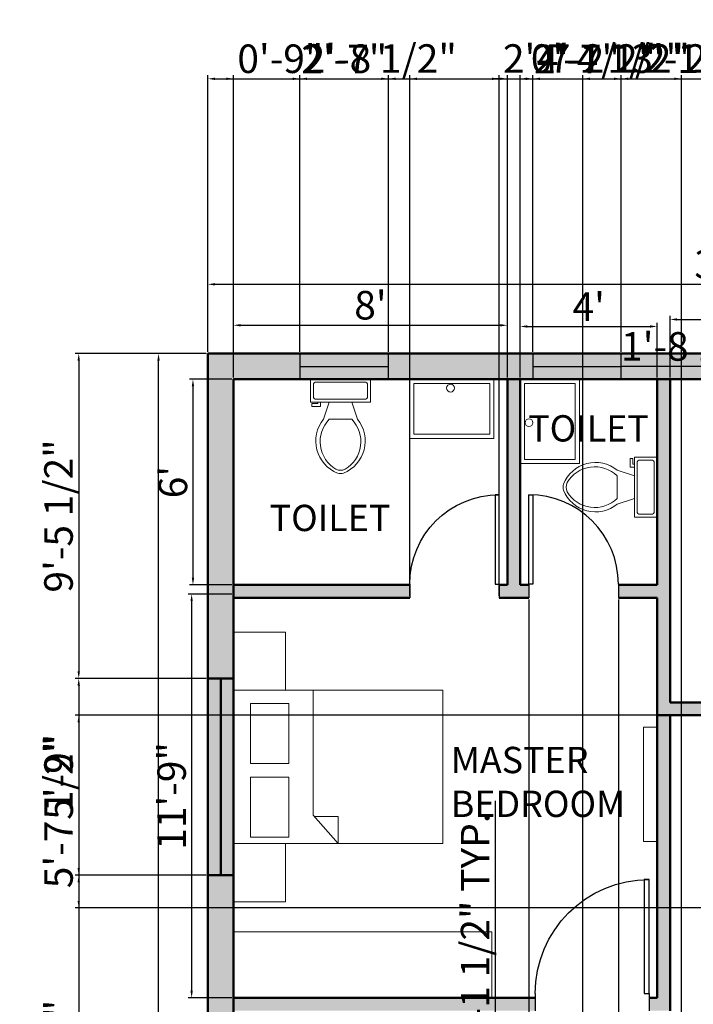
# Model space of a CAD drawing. Units: inches. Extents: x 1344 to 2521, y 3236 to 4924.
# Tile 11 of 14: x 1348 to 1584, y 4525 to 4870. Entities that reach past the tile are written whole.
import ezdxf

# ---------------------------------------------------------------- set-up
doc = ezdxf.new("R2010")
doc.units = ezdxf.units.IN
for name, color, linetype, lineweight in [('A-ANNO-DIMS', 2, 'Continuous', 18), ('A-AREA-IDEN', 3, 'Continuous', 18), ('A-DOOR', 50, 'Continuous', 25), ('A-FLOR-FIXT', 8, 'Continuous', 18), ('A-FURN', 130, 'Continuous', 18), ('A-GLAZ', 150, 'Continuous', 25), ('A-WALL', 31, 'Continuous', 50), ('A-WALL-PATT', 8, 'Continuous', 13)]:
    doc.layers.add(name, color=color, linetype=linetype, lineweight=lineweight)
doc.styles.get("Standard").update_dxf_attribs({"font": 'arial.ttf'})
doc.dimstyles.new('ISO-25', dxfattribs={"dimtxt": 10, "dimasz": 2.5, "dimexe": 1.25, "dimexo": 0.625, "dimtad": 1, "dimdec": 0, "dimlunit": 4, "dimtxsty": 'Standard', "dimcen": 2.5, "dimadec": 0, "dimazin": 0, "dimtfac": 1, "dimtdec": 0, "dimtmove": 0, "dimatfit": 3, "dimfxl": 1, "dimarcsym": 0})

# ---------------------------------------------------------------- blocks, each defined once
blk = doc.blocks.new('*U6')
for p, q in [((9.5, -6), (9.5, -2)), ((-10, -8.5), (-8, -8.5)), ((-10, -9.5), (-10, -8.5)), ((-7, -9.5), (-10, -9.5)), ((-8, -8.5), (-8, -8)), ((-7, -8), (-7, -9.5)), ((-4, -8), (-6, -14)), ((4, -8), (6, -14)), ((4, -14), (-4, -14))]:
    blk.add_line(p, q)
blk.add_lwpolyline([(10.5, -8), (10.5, 0), (-10.5, 0), (-10.5, -8)], close=True)
for points in [[(-9.5, -2), (-9.5, -6)], [(8.5, -1), (-8.5, -1)], [(-8.5, -7), (8.5, -7)]]:
    blk.add_lwpolyline(points)
for centre, radius, start, end in [((-8.62, -1.88), 0.884, 81.8699, 188.1301), ((8.62, -1.88), 0.884, 351.8699, 98.1301), ((-8.62, -6.12), 0.884, 171.8699, 278.1301), ((8.62, -6.12), 0.884, 261.8699, 8.1301), ((3.52, -21.58), 12.17, 141.4691, 247.9714), ((4.2, -21.82), 11.33, 136.3677, 238.9468), ((-3.52, -21.58), 12.17, 292.0284, 38.5307), ((-4.2, -21.82), 11.33, 301.053, 43.6321), ((0, -27.88), 4, 245.7318, 294.2682), ((0, -29), 4, 254.8605, 285.1395)]:
    blk.add_arc(centre, radius, start, end)
blk = doc.blocks.new('*U2')
for p, q in [((0, 0), (0, -6)), ((40, 0), (40, -6))]:
    blk.add_line(p, q)
blk.add_lwpolyline([(0, 0), (0, 40), (1.75, 40), (1.75, 0)], close=True)
blk.add_arc((0, 0), 40, 0, 90)
blk = doc.blocks.new('*D15')
at = {"layer": 'A-ANNO-DIMS', "color": 0, "lineweight": -2, "transparency": 16777216}
for p, q in [((1413.52, 4753.84), (1413.52, 4778.73)), ((1416.02, 4777.48), (1771.02, 4777.48)), ((1773.52, 4753.84), (1773.52, 4778.73))]:
    blk.add_line(p, q, dxfattribs=at)
at = {"layer": 'A-ANNO-DIMS', "color": 0, "lineweight": 100, "transparency": 16777216}
for points in [[(1416.02, 4777.9), (1416.02, 4777.06), (1413.52, 4777.48)], [(1771.02, 4777.9), (1771.02, 4777.06), (1773.52, 4777.48)]]:
    blk.add_solid(points, dxfattribs=at)
at = {"layer": 'Defpoints', "color": 0, "lineweight": 100, "transparency": 16777216}
for p in [(1773.52, 4777.48), (1413.52, 4753.21), (1773.52, 4753.21)]:
    blk.add_point(p, dxfattribs=at)
at = {"layer": 'A-ANNO-DIMS', "color": 0, "transparency": 16777216, "insert": (1593.52, 4783.21), "char_height": 10, "attachment_point": 5}
blk.add_mtext("30'", dxfattribs=at)
blk = doc.blocks.new('*D16')
at = {"layer": 'A-ANNO-DIMS', "color": 0, "lineweight": -2, "transparency": 16777216}
for p, q in [((1412.89, 4753.21), (1394.98, 4753.21)), ((1396.23, 4155.71), (1396.23, 4750.71)), ((1412.89, 4153.21), (1394.98, 4153.21))]:
    blk.add_line(p, q, dxfattribs=at)
at = {"layer": 'A-ANNO-DIMS', "color": 0, "lineweight": 100, "transparency": 16777216}
for points in [[(1395.81, 4750.71), (1396.65, 4750.71), (1396.23, 4753.21)], [(1395.81, 4155.71), (1396.65, 4155.71), (1396.23, 4153.21)]]:
    blk.add_solid(points, dxfattribs=at)
at = {"layer": 'Defpoints', "color": 0, "lineweight": 100, "transparency": 16777216}
for p in [(1396.23, 4753.21), (1413.52, 4753.21), (1413.52, 4153.21)]:
    blk.add_point(p, dxfattribs=at)
at = {"layer": 'A-ANNO-DIMS', "color": 0, "transparency": 16777216, "insert": (1390.5, 4453.21), "char_height": 10, "attachment_point": 5, "rotation": 90}
blk.add_mtext("50'", dxfattribs=at)
blk = doc.blocks.new('*D17')
at = {"layer": 'A-ANNO-DIMS', "color": 0, "lineweight": -2, "transparency": 16777216}
for p, q in [((1422.52, 4744.84), (1422.52, 4764.39)), ((1425.02, 4763.14), (1516.02, 4763.14)), ((1518.52, 4744.84), (1518.52, 4764.39))]:
    blk.add_line(p, q, dxfattribs=at)
at = {"layer": 'A-ANNO-DIMS', "color": 0, "lineweight": 100, "transparency": 16777216}
for points in [[(1425.02, 4763.55), (1425.02, 4762.72), (1422.52, 4763.14)], [(1516.02, 4763.55), (1516.02, 4762.72), (1518.52, 4763.14)]]:
    blk.add_solid(points, dxfattribs=at)
at = {"layer": 'Defpoints', "color": 0, "lineweight": 100, "transparency": 16777216}
for p in [(1518.52, 4763.14), (1422.52, 4744.21), (1518.52, 4744.21)]:
    blk.add_point(p, dxfattribs=at)
at = {"layer": 'A-ANNO-DIMS', "color": 0, "transparency": 16777216, "insert": (1470.52, 4768.87), "char_height": 10, "attachment_point": 5}
blk.add_mtext("8'", dxfattribs=at)
blk = doc.blocks.new('*D18')
at = {"layer": 'A-ANNO-DIMS', "color": 0, "lineweight": -2, "transparency": 16777216}
for p, q in [((1523.02, 4744.84), (1523.02, 4763.97)), ((1525.52, 4762.72), (1568.52, 4762.72)), ((1571.02, 4744.84), (1571.02, 4763.97))]:
    blk.add_line(p, q, dxfattribs=at)
at = {"layer": 'A-ANNO-DIMS', "color": 0, "lineweight": 100, "transparency": 16777216}
for points in [[(1525.52, 4763.14), (1525.52, 4762.3), (1523.02, 4762.72)], [(1568.52, 4763.14), (1568.52, 4762.3), (1571.02, 4762.72)]]:
    blk.add_solid(points, dxfattribs=at)
at = {"layer": 'Defpoints', "color": 0, "lineweight": 100, "transparency": 16777216}
for p in [(1571.02, 4762.72), (1523.02, 4744.21), (1571.02, 4744.21)]:
    blk.add_point(p, dxfattribs=at)
at = {"layer": 'A-ANNO-DIMS', "color": 0, "transparency": 16777216, "insert": (1547.02, 4768.34), "char_height": 10, "attachment_point": 5}
blk.add_mtext("4'", dxfattribs=at)
blk = doc.blocks.new('*D19')
at = {"layer": 'A-ANNO-DIMS', "color": 0, "lineweight": -2, "transparency": 16777216}
for p, q in [((1575.52, 4744.84), (1575.52, 4766.43)), ((1640.94, 4744.84), (1640.94, 4766.43)), ((1578.02, 4765.18), (1638.44, 4765.18))]:
    blk.add_line(p, q, dxfattribs=at)
at = {"layer": 'A-ANNO-DIMS', "color": 0, "lineweight": 100, "transparency": 16777216}
for points in [[(1578.02, 4765.59), (1578.02, 4764.76), (1575.52, 4765.18)], [(1638.44, 4765.59), (1638.44, 4764.76), (1640.94, 4765.18)]]:
    blk.add_solid(points, dxfattribs=at)
at = {"layer": 'Defpoints', "color": 0, "lineweight": 100, "transparency": 16777216}
for p in [(1640.94, 4765.18), (1575.52, 4744.21), (1640.94, 4744.21)]:
    blk.add_point(p, dxfattribs=at)
at = {"layer": 'A-ANNO-DIMS', "color": 0, "transparency": 16777216, "insert": (1608.23, 4770.89), "char_height": 10, "attachment_point": 5}
blk.add_mtext('5\'-5"', dxfattribs=at)
blk = doc.blocks.new('*D21')
at = {"layer": 'A-ANNO-DIMS', "color": 0, "lineweight": -2, "transparency": 16777216}
for p, q in [((1421.89, 4744.21), (1407.05, 4744.21)), ((1408.3, 4741.71), (1408.3, 4674.71)), ((1421.89, 4672.21), (1407.05, 4672.21))]:
    blk.add_line(p, q, dxfattribs=at)
at = {"layer": 'A-ANNO-DIMS', "color": 0, "lineweight": 100, "transparency": 16777216}
for points in [[(1407.89, 4741.71), (1408.72, 4741.71), (1408.3, 4744.21)], [(1407.89, 4674.71), (1408.72, 4674.71), (1408.3, 4672.21)]]:
    blk.add_solid(points, dxfattribs=at)
at = {"layer": 'Defpoints', "color": 0, "lineweight": 100, "transparency": 16777216}
for p in [(1422.52, 4744.21), (1408.3, 4672.21), (1422.52, 4672.21)]:
    blk.add_point(p, dxfattribs=at)
at = {"layer": 'A-ANNO-DIMS', "color": 0, "transparency": 16777216, "insert": (1402.57, 4708.21), "char_height": 10, "attachment_point": 5, "rotation": 90}
blk.add_mtext("6'", dxfattribs=at)
blk = doc.blocks.new('*D22')
at = {"layer": 'A-ANNO-DIMS', "color": 0, "lineweight": -2, "transparency": 16777216}
for p, q in [((1421.89, 4669), (1406.59, 4669)), ((1407.84, 4666.5), (1407.84, 4530.04)), ((1421.89, 4527.54), (1406.59, 4527.54))]:
    blk.add_line(p, q, dxfattribs=at)
at = {"layer": 'A-ANNO-DIMS', "color": 0, "lineweight": 100, "transparency": 16777216}
for points in [[(1407.42, 4666.5), (1408.25, 4666.5), (1407.84, 4669)], [(1407.42, 4530.04), (1408.25, 4530.04), (1407.84, 4527.54)]]:
    blk.add_solid(points, dxfattribs=at)
at = {"layer": 'Defpoints', "color": 0, "lineweight": 100, "transparency": 16777216}
for p in [(1422.52, 4669), (1407.84, 4527.54), (1422.52, 4527.54)]:
    blk.add_point(p, dxfattribs=at)
at = {"layer": 'A-ANNO-DIMS', "color": 0, "transparency": 16777216, "insert": (1402.11, 4598.27), "char_height": 10, "attachment_point": 5, "rotation": 90}
blk.add_mtext('11\'-9"', dxfattribs=at)
blk = doc.blocks.new('BED-DOUBLE')
for p, q in [((27.95, 53.78), (27.95, 9.98)), ((27.95, 9.98), (36.68, 0)), ((36.68, 9.56), (28.32, 9.56)), ((36.68, 0), (36.68, 9.56))]:
    blk.add_line(p, q)
for points in [[(0, 0), (73.35, 0), (73.35, 53.78), (0, 53.78)], [(5.91, 28.08), (19.39, 28.08), (19.39, 49.13), (5.91, 49.13)], [(5.91, 2.27), (19.39, 2.27), (19.39, 23.31), (5.91, 23.31)]]:
    blk.add_lwpolyline(points, close=True)
blk = doc.blocks.new('WASH-BASIN')
for points in [[(29.51, 20.73), (0, 20.73), (0, 0), (29.51, 0)], [(28.05, 19.27), (1.46, 19.27), (1.46, 1.46), (28.05, 1.46)]]:
    blk.add_lwpolyline(points, close=True)
blk.add_circle((14.31, 17.66), 1.38)
blk = doc.blocks.new('*D63')
at = {"layer": 'A-ANNO-DIMS', "color": 0, "lineweight": -2, "transparency": 16777216}
for p, q in [((1514.3, 4415.14), (1514.3, 4596.59)), ((1503.92, 4415.14), (1515.55, 4415.14)), ((1514.3, 4344.29), (1514.3, 4412.64)), ((1503.92, 4341.79), (1515.55, 4341.79))]:
    blk.add_line(p, q, dxfattribs=at)
at = {"layer": 'A-ANNO-DIMS', "color": 0, "lineweight": 100, "transparency": 16777216}
for points in [[(1513.88, 4412.64), (1514.72, 4412.64), (1514.3, 4415.14)], [(1513.88, 4344.29), (1514.72, 4344.29), (1514.3, 4341.79)]]:
    blk.add_solid(points, dxfattribs=at)
at = {"layer": 'Defpoints', "color": 0, "lineweight": 100, "transparency": 16777216}
for p in [(1503.3, 4415.14), (1514.3, 4415.14), (1503.3, 4341.79)]:
    blk.add_point(p, dxfattribs=at)
at = {"layer": 'A-ANNO-DIMS', "color": 0, "transparency": 16777216, "insert": (1508.5, 4507.12), "char_height": 10, "attachment_point": 5, "rotation": 90}
blk.add_mtext('DOUBLE BED 6\'-1 1/2" TYP.', dxfattribs=at)
blk = doc.blocks.new('*D66')
at = {"layer": 'A-ANNO-DIMS', "color": 0, "lineweight": -2, "transparency": 16777216}
for p, q in [((1645.44, 4744.84), (1645.44, 4749.89)), ((1666.17, 4744.84), (1666.17, 4749.89)), ((1645.44, 4748.64), (1558.38, 4748.64)), ((1663.67, 4748.64), (1647.94, 4748.64))]:
    blk.add_line(p, q, dxfattribs=at)
at = {"layer": 'A-ANNO-DIMS', "color": 0, "lineweight": 100, "transparency": 16777216}
for points in [[(1647.94, 4749.05), (1647.94, 4748.22), (1645.44, 4748.64)], [(1663.67, 4749.05), (1663.67, 4748.22), (1666.17, 4748.64)]]:
    blk.add_solid(points, dxfattribs=at)
at = {"layer": 'Defpoints', "color": 0, "lineweight": 100, "transparency": 16777216}
for p in [(1645.44, 4748.64), (1645.44, 4744.21), (1666.17, 4744.21)]:
    blk.add_point(p, dxfattribs=at)
at = {"layer": 'A-ANNO-DIMS', "color": 0, "transparency": 16777216, "insert": (1600.66, 4754.43), "char_height": 10, "attachment_point": 5}
blk.add_mtext('1\'-8 1/2" TYP.', dxfattribs=at)
blk = doc.blocks.new('*D69')
at = {"layer": 'A-ANNO-DIMS', "color": 0, "lineweight": -2, "transparency": 16777216}
for p, q in [((1413.52, 4753.84), (1413.52, 4850.71)), ((1416.02, 4849.46), (1420.02, 4849.46)), ((1422.52, 4744.84), (1422.52, 4850.71)), ((1422.52, 4849.46), (1452.85, 4849.46))]:
    blk.add_line(p, q, dxfattribs=at)
at = {"layer": 'A-ANNO-DIMS', "color": 0, "lineweight": 100, "transparency": 16777216}
for points in [[(1416.02, 4849.88), (1416.02, 4849.04), (1413.52, 4849.46)], [(1420.02, 4849.88), (1420.02, 4849.04), (1422.52, 4849.46)]]:
    blk.add_solid(points, dxfattribs=at)
at = {"layer": 'Defpoints', "color": 0, "lineweight": 100, "transparency": 16777216}
for p in [(1422.52, 4849.46), (1413.52, 4753.21), (1422.52, 4744.21)]:
    blk.add_point(p, dxfattribs=at)
at = {"layer": 'A-ANNO-DIMS', "color": 0, "transparency": 16777216, "insert": (1438.93, 4855.19), "char_height": 10, "attachment_point": 5}
blk.add_mtext('0\'-9"', dxfattribs=at)
blk = doc.blocks.new('*D70')
at = {"layer": 'A-ANNO-DIMS', "color": 0, "lineweight": -2, "transparency": 16777216}
for p, q in [((1516.02, 4849.46), (1513.52, 4849.46)), ((1518.52, 4744.84), (1518.52, 4850.71)), ((1518.52, 4849.46), (1523.02, 4849.46)), ((1523.02, 4744.84), (1523.02, 4850.71)), ((1525.52, 4849.46), (1579.15, 4849.46))]:
    blk.add_line(p, q, dxfattribs=at)
at = {"layer": 'A-ANNO-DIMS', "color": 0, "lineweight": 100, "transparency": 16777216}
for points in [[(1516.02, 4849.88), (1516.02, 4849.04), (1518.52, 4849.46)], [(1525.52, 4849.88), (1525.52, 4849.04), (1523.02, 4849.46)]]:
    blk.add_solid(points, dxfattribs=at)
at = {"layer": 'Defpoints', "color": 0, "lineweight": 100, "transparency": 16777216}
for p in [(1523.02, 4849.46), (1518.52, 4744.21), (1523.02, 4744.21)]:
    blk.add_point(p, dxfattribs=at)
at = {"layer": 'A-ANNO-DIMS', "color": 0, "transparency": 16777216, "insert": (1553.58, 4855.26), "char_height": 10, "attachment_point": 5}
blk.add_mtext('0\'-4 1/2"', dxfattribs=at)
blk = doc.blocks.new('*D71')
at = {"layer": 'A-ANNO-DIMS', "color": 0, "lineweight": -2, "transparency": 16777216}
for p, q in [((1413.52, 4753.84), (1413.52, 4850.71)), ((1416.02, 4849.46), (1443.3, 4849.46)), ((1445.8, 4753.84), (1445.8, 4850.71)), ((1445.8, 4849.46), (1499.6, 4849.46))]:
    blk.add_line(p, q, dxfattribs=at)
at = {"layer": 'A-ANNO-DIMS', "color": 0, "lineweight": 100, "transparency": 16777216}
for points in [[(1416.02, 4849.88), (1416.02, 4849.04), (1413.52, 4849.46)], [(1443.3, 4849.88), (1443.3, 4849.04), (1445.8, 4849.46)]]:
    blk.add_solid(points, dxfattribs=at)
at = {"layer": 'Defpoints', "color": 0, "lineweight": 100, "transparency": 16777216}
for p in [(1445.8, 4849.46), (1413.52, 4753.21), (1445.8, 4753.21)]:
    blk.add_point(p, dxfattribs=at)
at = {"layer": 'A-ANNO-DIMS', "color": 0, "transparency": 16777216, "insert": (1473.95, 4855.26), "char_height": 10, "attachment_point": 5}
blk.add_mtext('2\'-8 1/2"', dxfattribs=at)
blk = doc.blocks.new('*D72')
at = {"layer": 'A-ANNO-DIMS', "color": 0, "lineweight": -2, "transparency": 16777216}
for p, q in [((1445.8, 4753.84), (1445.8, 4850.71)), ((1448.3, 4849.46), (1474.33, 4849.46)), ((1476.83, 4753.84), (1476.83, 4850.71))]:
    blk.add_line(p, q, dxfattribs=at)
at = {"layer": 'A-ANNO-DIMS', "color": 0, "lineweight": 100, "transparency": 16777216}
for points in [[(1448.3, 4849.88), (1448.3, 4849.04), (1445.8, 4849.46)], [(1474.33, 4849.88), (1474.33, 4849.04), (1476.83, 4849.46)]]:
    blk.add_solid(points, dxfattribs=at)
at = {"layer": 'Defpoints', "color": 0, "lineweight": 100, "transparency": 16777216}
for p in [(1476.83, 4849.46), (1445.8, 4753.21), (1476.83, 4753.21)]:
    blk.add_point(p, dxfattribs=at)
at = {"layer": 'A-ANNO-DIMS', "color": 0, "transparency": 16777216, "insert": (1461.31, 4855.11), "char_height": 10, "attachment_point": 5}
blk.add_mtext('2\'-7"', dxfattribs=at)
blk = doc.blocks.new('*D73')
at = {"layer": 'A-ANNO-DIMS', "color": 0, "lineweight": -2, "transparency": 16777216}
for p, q in [((1476.83, 4753.84), (1476.83, 4850.71)), ((1479.33, 4849.46), (1524.9, 4849.46)), ((1527.4, 4753.84), (1527.4, 4850.71)), ((1527.4, 4849.46), (1581.43, 4849.46))]:
    blk.add_line(p, q, dxfattribs=at)
at = {"layer": 'A-ANNO-DIMS', "color": 0, "lineweight": 100, "transparency": 16777216}
for points in [[(1479.33, 4849.88), (1479.33, 4849.04), (1476.83, 4849.46)], [(1524.9, 4849.88), (1524.9, 4849.04), (1527.4, 4849.46)]]:
    blk.add_solid(points, dxfattribs=at)
at = {"layer": 'Defpoints', "color": 0, "lineweight": 100, "transparency": 16777216}
for p in [(1527.4, 4849.46), (1476.83, 4753.21), (1527.4, 4753.21)]:
    blk.add_point(p, dxfattribs=at)
at = {"layer": 'A-ANNO-DIMS', "color": 0, "transparency": 16777216, "insert": (1555.66, 4855.26), "char_height": 10, "attachment_point": 5}
blk.add_mtext('4\'-2 1/2"', dxfattribs=at)
blk = doc.blocks.new('*D74')
at = {"layer": 'A-ANNO-DIMS', "color": 0, "lineweight": -2, "transparency": 16777216}
for p, q in [((1527.4, 4753.84), (1527.4, 4850.71)), ((1529.9, 4849.46), (1555.93, 4849.46)), ((1558.43, 4753.84), (1558.43, 4850.71))]:
    blk.add_line(p, q, dxfattribs=at)
at = {"layer": 'A-ANNO-DIMS', "color": 0, "lineweight": 100, "transparency": 16777216}
for points in [[(1529.9, 4849.88), (1529.9, 4849.04), (1527.4, 4849.46)], [(1555.93, 4849.88), (1555.93, 4849.04), (1558.43, 4849.46)]]:
    blk.add_solid(points, dxfattribs=at)
at = {"layer": 'Defpoints', "color": 0, "lineweight": 100, "transparency": 16777216}
for p in [(1558.43, 4849.46), (1527.4, 4753.21), (1558.43, 4753.21)]:
    blk.add_point(p, dxfattribs=at)
at = {"layer": 'A-ANNO-DIMS', "color": 0, "transparency": 16777216, "insert": (1542.91, 4855.11), "char_height": 10, "attachment_point": 5}
blk.add_mtext('2\'-7"', dxfattribs=at)
blk = doc.blocks.new('*D75')
at = {"layer": 'A-ANNO-DIMS', "color": 0, "lineweight": -2, "transparency": 16777216}
for p, q in [((1558.43, 4753.84), (1558.43, 4850.71)), ((1560.93, 4849.46), (1593.16, 4849.46)), ((1595.66, 4753.84), (1595.66, 4850.71))]:
    blk.add_line(p, q, dxfattribs=at)
at = {"layer": 'A-ANNO-DIMS', "color": 0, "lineweight": 100, "transparency": 16777216}
for points in [[(1560.93, 4849.88), (1560.93, 4849.04), (1558.43, 4849.46)], [(1593.16, 4849.88), (1593.16, 4849.04), (1595.66, 4849.46)]]:
    blk.add_solid(points, dxfattribs=at)
at = {"layer": 'Defpoints', "color": 0, "lineweight": 100, "transparency": 16777216}
for p in [(1595.66, 4849.46), (1558.43, 4753.21), (1595.66, 4753.21)]:
    blk.add_point(p, dxfattribs=at)
at = {"layer": 'A-ANNO-DIMS', "color": 0, "transparency": 16777216, "insert": (1577.04, 4855.2), "char_height": 10, "attachment_point": 5}
blk.add_mtext('3\'-1"', dxfattribs=at)
blk = doc.blocks.new('*D80')
at = {"layer": 'A-ANNO-DIMS', "color": 0, "lineweight": -2, "transparency": 16777216}
for p, q in [((1412.89, 4753.21), (1367.02, 4753.21)), ((1368.27, 4750.71), (1368.27, 4641.96)), ((1412.89, 4639.46), (1367.02, 4639.46))]:
    blk.add_line(p, q, dxfattribs=at)
at = {"layer": 'A-ANNO-DIMS', "color": 0, "lineweight": 100, "transparency": 16777216}
for points in [[(1367.85, 4750.71), (1368.68, 4750.71), (1368.27, 4753.21)], [(1367.85, 4641.96), (1368.68, 4641.96), (1368.27, 4639.46)]]:
    blk.add_solid(points, dxfattribs=at)
at = {"layer": 'Defpoints', "color": 0, "lineweight": 100, "transparency": 16777216}
for p in [(1413.52, 4753.21), (1368.27, 4639.46), (1413.52, 4639.46)]:
    blk.add_point(p, dxfattribs=at)
at = {"layer": 'A-ANNO-DIMS', "color": 0, "transparency": 16777216, "insert": (1362.47, 4696.34), "char_height": 10, "attachment_point": 5, "rotation": 90}
blk.add_mtext('9\'-5 1/2"', dxfattribs=at)
blk = doc.blocks.new('*D81')
at = {"layer": 'A-ANNO-DIMS', "color": 0, "lineweight": -2, "transparency": 16777216}
for p, q in [((1412.89, 4639.46), (1367.02, 4639.46)), ((1368.27, 4636.96), (1368.27, 4573.04)), ((1412.89, 4570.54), (1367.02, 4570.54))]:
    blk.add_line(p, q, dxfattribs=at)
at = {"layer": 'A-ANNO-DIMS', "color": 0, "lineweight": 100, "transparency": 16777216}
for points in [[(1367.85, 4636.96), (1368.68, 4636.96), (1368.27, 4639.46)], [(1367.85, 4573.04), (1368.68, 4573.04), (1368.27, 4570.54)]]:
    blk.add_solid(points, dxfattribs=at)
at = {"layer": 'Defpoints', "color": 0, "lineweight": 100, "transparency": 16777216}
for p in [(1413.52, 4639.46), (1368.27, 4570.54), (1413.52, 4570.54)]:
    blk.add_point(p, dxfattribs=at)
at = {"layer": 'A-ANNO-DIMS', "color": 0, "transparency": 16777216, "insert": (1362.54, 4605), "char_height": 10, "attachment_point": 5, "rotation": 90}
blk.add_mtext('5\'-9"', dxfattribs=at)
blk = doc.blocks.new('*D82')
at = {"layer": 'A-ANNO-DIMS', "color": 0, "lineweight": -2, "transparency": 16777216}
for p, q in [((1412.89, 4570.54), (1367.02, 4570.54)), ((1368.27, 4568.04), (1368.27, 4448.1)), ((1412.89, 4445.6), (1367.02, 4445.6))]:
    blk.add_line(p, q, dxfattribs=at)
at = {"layer": 'A-ANNO-DIMS', "color": 0, "lineweight": 100, "transparency": 16777216}
for points in [[(1367.85, 4568.04), (1368.68, 4568.04), (1368.27, 4570.54)], [(1367.85, 4448.1), (1368.68, 4448.1), (1368.27, 4445.6)]]:
    blk.add_solid(points, dxfattribs=at)
at = {"layer": 'Defpoints', "color": 0, "lineweight": 100, "transparency": 16777216}
for p in [(1413.52, 4570.54), (1368.27, 4445.6), (1413.52, 4445.6)]:
    blk.add_point(p, dxfattribs=at)
at = {"layer": 'A-ANNO-DIMS', "color": 0, "transparency": 16777216, "insert": (1362.54, 4508.07), "char_height": 10, "attachment_point": 5, "rotation": 90}
blk.add_mtext('10\'-5"', dxfattribs=at)
blk = doc.blocks.new('*D92')
at = {"layer": 'A-ANNO-DIMS', "color": 0, "lineweight": -2, "transparency": 16777216}
for p, q in [((1484.28, 4668.34), (1484.28, 4850.71)), ((1486.78, 4849.46), (1513.16, 4849.46)), ((1515.66, 4668.34), (1515.66, 4850.71)), ((1515.66, 4849.46), (1569.47, 4849.46))]:
    blk.add_line(p, q, dxfattribs=at)
at = {"layer": 'A-ANNO-DIMS', "color": 0, "lineweight": 100, "transparency": 16777216}
for points in [[(1486.78, 4849.88), (1486.78, 4849.04), (1484.28, 4849.46)], [(1513.16, 4849.88), (1513.16, 4849.04), (1515.66, 4849.46)]]:
    blk.add_solid(points, dxfattribs=at)
at = {"layer": 'Defpoints', "color": 0, "lineweight": 100, "transparency": 16777216}
for p in [(1515.66, 4849.46), (1484.28, 4667.71), (1515.66, 4667.71)]:
    blk.add_point(p, dxfattribs=at)
at = {"layer": 'A-ANNO-DIMS', "color": 0, "transparency": 16777216, "insert": (1543.81, 4855.26), "char_height": 10, "attachment_point": 5}
blk.add_mtext('2\'-7 1/2"', dxfattribs=at)
blk = doc.blocks.new('*D93')
at = {"layer": 'A-ANNO-DIMS', "color": 0, "lineweight": -2, "transparency": 16777216}
for p, q in [((1526.04, 4667.09), (1526.04, 4106.71)), ((1557.42, 4667.09), (1557.42, 4106.71)), ((1528.54, 4107.96), (1554.92, 4107.96)), ((1557.42, 4107.96), (1611.23, 4107.96))]:
    blk.add_line(p, q, dxfattribs=at)
at = {"layer": 'A-ANNO-DIMS', "color": 0, "lineweight": 100, "transparency": 16777216}
for points in [[(1528.54, 4108.38), (1528.54, 4107.54), (1526.04, 4107.96)], [(1554.92, 4108.38), (1554.92, 4107.54), (1557.42, 4107.96)]]:
    blk.add_solid(points, dxfattribs=at)
at = {"layer": 'Defpoints', "color": 0, "lineweight": 100, "transparency": 16777216}
for p in [(1526.04, 4667.71), (1557.42, 4667.71), (1557.42, 4107.96)]:
    blk.add_point(p, dxfattribs=at)
at = {"layer": 'A-ANNO-DIMS', "color": 0, "transparency": 16777216, "insert": (1585.57, 4113.76), "char_height": 10, "attachment_point": 5}
blk.add_mtext('2\'-7 1/2"', dxfattribs=at)
blk = doc.blocks.new('*D96')
at = {"layer": 'A-ANNO-DIMS', "color": 0, "lineweight": -2, "transparency": 16777216}
for p, q in [((1644.82, 4626.56), (1367.02, 4626.56)), ((1368.27, 4624.06), (1368.27, 4561.53)), ((1640.32, 4559.03), (1367.02, 4559.03))]:
    blk.add_line(p, q, dxfattribs=at)
at = {"layer": 'A-ANNO-DIMS', "color": 0, "lineweight": 100, "transparency": 16777216}
for points in [[(1367.85, 4624.06), (1368.68, 4624.06), (1368.27, 4626.56)], [(1367.85, 4561.53), (1368.68, 4561.53), (1368.27, 4559.03)]]:
    blk.add_solid(points, dxfattribs=at)
at = {"layer": 'Defpoints', "color": 0, "lineweight": 100, "transparency": 16777216}
for p in [(1645.44, 4626.56), (1368.27, 4559.03), (1640.94, 4559.03)]:
    blk.add_point(p, dxfattribs=at)
at = {"layer": 'A-ANNO-DIMS', "color": 0, "transparency": 16777216, "insert": (1362.47, 4592.79), "char_height": 10, "attachment_point": 5, "rotation": 90}
blk.add_mtext('5\'-7 1/2"', dxfattribs=at)
blk = doc.blocks.new('*D99')
at = {"layer": 'A-ANNO-DIMS', "color": 0, "lineweight": -2, "transparency": 16777216}
for p, q in [((1544.94, 4337.92), (1544.94, 4850.71)), ((1547.44, 4849.46), (1577, 4849.46)), ((1579.5, 4337.92), (1579.5, 4850.71)), ((1579.5, 4849.46), (1641.07, 4849.46))]:
    blk.add_line(p, q, dxfattribs=at)
at = {"layer": 'A-ANNO-DIMS', "color": 0, "lineweight": 100, "transparency": 16777216}
for points in [[(1547.44, 4849.88), (1547.44, 4849.04), (1544.94, 4849.46)], [(1577, 4849.88), (1577, 4849.04), (1579.5, 4849.46)]]:
    blk.add_solid(points, dxfattribs=at)
at = {"layer": 'Defpoints', "color": 0, "lineweight": 100, "transparency": 16777216}
for p in [(1579.5, 4849.46), (1544.94, 4337.29), (1579.5, 4337.29)]:
    blk.add_point(p, dxfattribs=at)
at = {"layer": 'A-ANNO-DIMS', "color": 0, "transparency": 16777216, "insert": (1611.53, 4855.26), "char_height": 10, "attachment_point": 5}
blk.add_mtext('2\'-10 1/2"', dxfattribs=at)

msp = doc.modelspace()

# ---------------------------------------------------------------- hatches: boundary and pattern name
at = {"layer": 'A-WALL-PATT'}
h = msp.add_hatch(color=256, dxfattribs=at)
h.dxf.hatch_style = 1
h.paths.add_polyline_path([(1595.66, 4753.21), (1558.43, 4753.21), (1558.43, 4744.21), (1571.02, 4744.21), (1595.66, 4744.21)])
h.paths.add_polyline_path([(1681.23, 4753.21), (1626.69, 4753.21), (1626.69, 4744.21), (1681.23, 4744.21)])
h.paths.add_polyline_path([(1773.52, 4753.21), (1712.26, 4753.21), (1712.26, 4744.21), (1764.52, 4744.21), (1764.52, 4629.08), (1773.52, 4629.08)])
h.paths.add_polyline_path([(1527.4, 4753.21), (1476.83, 4753.21), (1476.83, 4744.21), (1518.52, 4744.21), (1527.4, 4744.21)])
h.paths.add_polyline_path([(1445.8, 4753.21), (1413.52, 4753.21), (1413.52, 4639.46), (1422.52, 4639.46), (1422.52, 4744.21), (1445.8, 4744.21)])
h.paths.add_polyline_path([(1523.02, 4744.21), (1518.52, 4744.21), (1518.52, 4672.21), (1515.66, 4672.21), (1515.66, 4667.71), (1523.02, 4667.71), (1526.04, 4667.71), (1526.04, 4672.21), (1523.02, 4672.21)])
h.paths.add_polyline_path([(1575.52, 4744.21), (1571.02, 4744.21), (1571.02, 4672.21), (1557.42, 4672.21), (1557.42, 4667.71), (1571.02, 4667.71), (1571.02, 4626.56), (1590.95, 4626.56), (1590.95, 4631.06), (1575.52, 4631.06), (1575.52, 4667.71)])
h.paths.add_polyline_path([(1484.28, 4672.21), (1422.52, 4672.21), (1422.52, 4667.71), (1484.28, 4667.71)])
h.paths.add_polyline_path([(1645.44, 4673.7), (1640.94, 4673.7), (1640.94, 4631.06), (1626.4, 4631.06), (1626.4, 4626.56), (1645.44, 4626.56)])
h.paths.add_polyline_path([(1645.44, 4744.21), (1640.94, 4744.21), (1640.94, 4713.7), (1645.44, 4713.7)])
h.paths.add_polyline_path([(1764.52, 4671), (1645.44, 4671), (1645.44, 4666.5), (1764.52, 4666.5)])
h.paths.add_polyline_path([(1764.52, 4527.54), (1640.94, 4527.54), (1640.94, 4523.04), (1764.52, 4523.04)])
h.paths.add_polyline_path([(1645.44, 4555.81), (1645.44, 4559.03), (1640.94, 4559.03), (1640.94, 4527.54), (1645.44, 4527.54)])
h = msp.add_hatch(color=256, dxfattribs=at)
h.dxf.hatch_style = 1
h.paths.add_polyline_path([(1773.52, 4425.27), (1764.52, 4425.27), (1764.52, 4225.22), (1743.16, 4225.22), (1743.16, 4216.22), (1764.52, 4216.22), (1764.52, 4162.21), (1764.52, 4155.88), (1653.6, 4155.88), (1653.6, 4177.58), (1764.52, 4177.58), (1764.52, 4180.4), (1649.25, 4180.4), (1649.25, 4153.21), (1773.52, 4153.21)], flags=17)
h.paths.add_polyline_path([(1598.02, 4180.38), (1593.52, 4180.38), (1589.02, 4180.38), (1589.02, 4162.21), (1565.92, 4162.21), (1565.92, 4153.21), (1598.02, 4153.21)], flags=17)
h.paths.add_polyline_path([(1689.47, 4225.22), (1666.04, 4225.22), (1666.04, 4220.75), (1666.04, 4216.22), (1689.47, 4216.22)], flags=16)
h.paths.add_polyline_path([(1442.43, 4162.21), (1422.52, 4162.21), (1422.52, 4744.21), (1764.52, 4744.21), (1764.52, 4225.22), (1743.16, 4225.22), (1743.16, 4216.22), (1764.52, 4216.22), (1764.52, 4162.21), (1764.52, 4155.88), (1653.6, 4155.88), (1653.6, 4177.58), (1764.52, 4177.58), (1764.52, 4180.4), (1649.25, 4180.4), (1649.25, 4153.21), (1773.52, 4153.21), (1773.52, 4425.27), (1773.52, 4753.21), (1413.52, 4753.21), (1413.52, 4153.21), (1442.43, 4153.21)])
h.paths.add_polyline_path([(1648.69, 4179.48), (1724.08, 4179.48), (1724.08, 4213.98), (1648.69, 4213.98)], flags=25)
h.paths.add_polyline_path([(1609.51, 4245.39), (1659.17, 4245.39), (1659.17, 4264.37), (1609.51, 4264.37)], flags=25)
h.paths.add_polyline_path([(1618.52, 4270.74), (1667.67, 4270.74), (1667.67, 4305.24), (1618.52, 4305.24)], flags=25)
h.paths.add_polyline_path([(1563.46, 4499.55), (1651.73, 4499.55), (1651.73, 4518.53), (1563.46, 4518.53)], flags=25)
h.paths.add_polyline_path([(1439.72, 4433.21), (1521.54, 4433.21), (1521.54, 4467.71), (1439.72, 4467.71)], flags=25)
h.paths.add_polyline_path([(1651.43, 4581.89), (1735.04, 4581.89), (1735.04, 4616.38), (1651.43, 4616.38)], flags=25)
h.paths.add_polyline_path([(1495.42, 4585.56), (1566.53, 4585.56), (1566.53, 4620.06), (1495.42, 4620.06)], flags=25)
h.paths.add_polyline_path([(1677.05, 4699.47), (1729.56, 4699.47), (1729.56, 4718.45), (1677.05, 4718.45)], flags=25)
h.paths.add_polyline_path([(1581.37, 4669.39), (1626.01, 4669.39), (1626.01, 4703.88), (1581.37, 4703.88)], flags=25)
h.paths.add_polyline_path([(1523.21, 4717.23), (1572.85, 4717.23), (1572.85, 4736.21), (1523.21, 4736.21)], flags=25)
h.paths.add_polyline_path([(1432.59, 4685.86), (1482.24, 4685.86), (1482.24, 4704.84), (1432.59, 4704.84)], flags=25)
h = msp.add_hatch(color=256, dxfattribs=at)
h.dxf.hatch_style = 1
h.paths.add_polyline_path([(1528.27, 4527.54), (1422.52, 4527.54), (1422.52, 4523.04), (1499.65, 4523.04), (1528.27, 4523.04)])
h.paths.add_polyline_path([(1575.52, 4626.56), (1571.02, 4626.56), (1571.02, 4527.54), (1568.27, 4527.54), (1568.27, 4523.04), (1575.52, 4523.04)])
h.paths.add_polyline_path([(1413.52, 4445.6), (1422.52, 4445.6), (1422.52, 4570.54), (1413.52, 4570.54)])

# ---------------------------------------------------------------- linework, layer by layer
at = {"layer": 'A-FURN'}
for points in [[(1422.52, 4635.35), (1440.75, 4635.35), (1440.75, 4655.69), (1422.52, 4655.69)], [(1571.02, 4622.31), (1566.22, 4622.31), (1566.22, 4582.33), (1571.02, 4582.33)], [(1422.52, 4561.23), (1440.75, 4561.23), (1440.75, 4581.57), (1422.52, 4581.57)], [(1513.01, 4527.54), (1422.52, 4527.54), (1422.52, 4550.66), (1513.01, 4550.66)]]:
    msp.add_lwpolyline(points, close=True, dxfattribs=at)
at = {"layer": 'A-GLAZ'}
for p, q in [((1445.8, 4748.71), (1476.83, 4748.71)), ((1445.8, 4748.71), (1476.83, 4748.71)), ((1527.4, 4748.71), (1558.43, 4748.71))]:
    msp.add_line(p, q, dxfattribs=at)
msp.add_lwpolyline([(1445.8, 4753.21), (1445.8, 4744.21), (1476.83, 4744.21), (1476.83, 4753.21)], dxfattribs=at)
for points in [[(1445.8, 4744.21), (1476.83, 4744.21), (1476.83, 4753.21), (1445.8, 4753.21)], [(1527.4, 4744.21), (1558.43, 4744.21), (1558.43, 4753.21), (1527.4, 4753.21)]]:
    msp.add_lwpolyline(points, close=True, dxfattribs=at)
at = {"layer": 'A-WALL'}
for p, q in [((1422.52, 4744.21), (1518.52, 4744.21)), ((1518.52, 4744.21), (1518.52, 4672.21)), ((1523.02, 4744.21), (1523.02, 4672.21)), ((1523.02, 4744.21), (1571.02, 4744.21)), ((1571.02, 4744.21), (1571.02, 4672.21)), ((1575.52, 4744.21), (1575.52, 4667.71)), ((1484.28, 4672.21), (1422.52, 4672.21)), ((1518.52, 4672.21), (1515.66, 4672.21)), ((1518.52, 4672.21), (1515.66, 4672.21)), ((1526.04, 4672.21), (1523.02, 4672.21)), ((1571.02, 4672.21), (1557.42, 4672.21)), ((1484.28, 4667.71), (1422.52, 4667.71)), ((1523.02, 4667.71), (1515.66, 4667.71)), ((1526.04, 4667.71), (1523.02, 4667.71)), ((1571.02, 4667.71), (1557.42, 4667.71)), ((1571.02, 4667.71), (1571.02, 4626.56)), ((1575.52, 4667.71), (1575.52, 4631.06)), ((1418.02, 4570.54), (1418.02, 4639.46)), ((1590.95, 4631.06), (1575.52, 4631.06)), ((1571.02, 4626.56), (1571.02, 4527.54)), ((1590.95, 4626.56), (1571.02, 4626.56)), ((1575.52, 4626.56), (1575.52, 4523.04)), ((1528.27, 4527.54), (1422.52, 4527.54)), ((1571.02, 4527.54), (1568.27, 4527.54))]:
    msp.add_line(p, q, dxfattribs=at)
for points in [[(1565.92, 4153.21), (1773.52, 4153.21), (1773.52, 4753.21), (1413.52, 4753.21), (1413.52, 4153.21), (1442.43, 4153.21)], [(1764.52, 4225.22), (1764.52, 4744.21), (1422.52, 4744.21), (1422.52, 4162.21), (1442.43, 4162.21)]]:
    msp.add_lwpolyline(points, dxfattribs=at)
msp.add_lwpolyline([(1413.52, 4570.54), (1422.52, 4570.54), (1422.52, 4639.46), (1413.52, 4639.46)], close=True, dxfattribs=at)

# ---------------------------------------------------------------- block references
at = {"layer": 'A-DOOR', "yscale": 0.7845484865997748, "zscale": 0.7845484865997748}
for p, xscale in [((1515.66, 4672.42), -0.7845484865997748), ((1526.04, 4672.42), 0.7845484865997748)]:
    msp.add_blockref('*U2', p, dxfattribs=dict(at, xscale=xscale))
at = {"layer": 'A-DOOR', "xscale": -1}
msp.add_blockref('*U2', (1568.27, 4529.04), dxfattribs=at)
at = {"layer": 'A-FLOR-FIXT'}
for name, p in [('*U6', (1460.02, 4744.21)), ('WASH-BASIN', (1484.28, 4723.48))]:
    msp.add_blockref(name, p, dxfattribs=at)
for name, p, rotation in [('WASH-BASIN', (1543.75, 4714.71), 90.00000000000146), ('*U6', (1571.02, 4706.43), 270)]:
    msp.add_blockref(name, p, dxfattribs=dict(at, rotation=rotation))
at = {"layer": 'A-FURN'}
msp.add_blockref('BED-DOUBLE', (1422.52, 4581.57), dxfattribs=at)

# ---------------------------------------------------------------- texts
at = {"layer": 'A-AREA-IDEN', "char_height": 9.211, "attachment_point": 1}
for s, insert in [('TOILET', (1525.81, 4731.63)), ('TOILET', (1435.19, 4700.26)), ('MASTER BEDROOM', (1498.68, 4615.47))]:
    msp.add_mtext_dynamic_manual_height_columns(s, width=108.7809, gutter_width=46.06, heights=[0], dxfattribs=dict(at, insert=insert))

# ---------------------------------------------------------------- dimensions: what is measured, and where the dimension line sits
at = {"layer": 'A-ANNO-DIMS'}
for base, p1, p2, override, picture, middle in [((1445.8, 4849.46), (1413.52, 4753.21), (1445.8, 4753.21), {"dimdec": 1, "dimlfac": 1, "dimrnd": 0, "dimzin": 1, "dimdsep": 46, "dimlunit": 4, "dimfrac": 2}, '*D71', (1473.95, 4855.26)), ((1527.4, 4849.46), (1476.83, 4753.21), (1527.4, 4753.21), {"dimdec": 1, "dimlfac": 1, "dimrnd": 0, "dimzin": 1, "dimdsep": 46, "dimlunit": 4, "dimfrac": 2}, '*D73', (1555.66, 4855.26)), ((1515.66, 4849.46), (1484.28, 4667.71), (1515.66, 4667.71), {"dimdec": 1, "dimlfac": 1, "dimrnd": 0, "dimzin": 1, "dimdsep": 46, "dimlunit": 4, "dimfrac": 2}, '*D92', (1543.81, 4855.26)), ((1523.02, 4849.46), (1518.52, 4744.21), (1523.02, 4744.21), {"dimdec": 1, "dimlfac": 1, "dimrnd": 0, "dimzin": 1, "dimdsep": 46, "dimlunit": 4, "dimfrac": 2}, '*D70', (1553.58, 4855.26)), ((1579.5, 4849.46), (1544.94, 4337.29), (1579.5, 4337.29), {"dimdec": 1, "dimlfac": 1, "dimrnd": 0, "dimzin": 1, "dimdsep": 46, "dimlunit": 4, "dimfrac": 2}, '*D99', (1611.53, 4855.26)), ((1422.52, 4849.46), (1413.52, 4753.21), (1422.52, 4744.21), {"dimdec": 1, "dimlfac": 1, "dimrnd": 0, "dimzin": 1, "dimdsep": 46, "dimlunit": 4, "dimfrac": 2}, '*D69', (1438.93, 4855.19)), ((1476.83, 4849.46), (1445.8, 4753.21), (1476.83, 4753.21), {"dimdec": 1, "dimlfac": 1, "dimrnd": 0, "dimzin": 1, "dimdsep": 46, "dimlunit": 4, "dimfrac": 2}, '*D72', (1461.31, 4855.11)), ((1558.43, 4849.46), (1527.4, 4753.21), (1558.43, 4753.21), {"dimdec": 1, "dimlfac": 1, "dimrnd": 0, "dimzin": 1, "dimdsep": 46, "dimlunit": 4, "dimfrac": 2}, '*D74', (1542.91, 4855.11)), ((1595.66, 4849.46), (1558.43, 4753.21), (1595.66, 4753.21), {"dimdec": 1, "dimlfac": 1, "dimrnd": 0, "dimzin": 1, "dimdsep": 46, "dimlunit": 4, "dimfrac": 2}, '*D75', (1577.04, 4855.2)), ((1773.52, 4777.48), (1413.52, 4753.21), (1773.52, 4753.21), {"dimclrd": 0, "dimclre": 0, "dimclrt": 0}, '*D15', (1593.52, 4783.21)), ((1640.94, 4765.18), (1575.52, 4744.21), (1640.94, 4744.21), {"dimclrd": 0, "dimclre": 0, "dimclrt": 0}, '*D19', (1608.23, 4770.89)), ((1518.52, 4763.14), (1422.52, 4744.21), (1518.52, 4744.21), {"dimclrd": 0, "dimclre": 0, "dimclrt": 0}, '*D17', (1470.52, 4768.87)), ((1571.02, 4762.72), (1523.02, 4744.21), (1571.02, 4744.21), {"dimclrd": 0, "dimclre": 0, "dimclrt": 0}, '*D18', (1547.02, 4768.34)), ((1557.42, 4107.96), (1526.04, 4667.71), (1557.42, 4667.71), {"dimdec": 1, "dimlfac": 1, "dimrnd": 0, "dimzin": 1, "dimdsep": 46, "dimlunit": 4, "dimfrac": 2}, '*D93', (1585.57, 4113.76))]:
    dim = msp.add_linear_dim(base=base, p1=p1, p2=p2, dimstyle='ISO-25', override=override, dxfattribs=at)
    dim.commit()
    dim.dimension.update_dxf_attribs({"geometry": picture, "text_midpoint": middle})
for base, p1, p2, angle, text, picture, middle in [((1645.44, 4748.64), (1666.17, 4744.21), (1645.44, 4744.21), 180, '<> TYP.', '*D66', (1600.66, 4754.43)), ((1514.2998, 4415.1429), (1503.2969, 4341.7902), (1503.2969, 4415.1429), 90, 'DOUBLE BED <> TYP.', '*D63', (1508.5009, 4507.1151))]:
    dim = msp.add_linear_dim(base=base, p1=p1, p2=p2, angle=angle, text=text, dimstyle='ISO-25', override={"dimdec": 1, "dimrnd": 0, "dimzin": 1, "dimlunit": 4, "dimfrac": 2}, dxfattribs=at)
    dim.commit()
    dim.dimension.update_dxf_attribs({"geometry": picture, "text_midpoint": middle})
for base, p1, p2, override, picture, middle in [((1368.2678, 4639.4624), (1413.5178, 4753.2109), (1413.5178, 4639.4624), {"dimdec": 1, "dimlfac": 1, "dimrnd": 0, "dimzin": 1, "dimdsep": 46, "dimlunit": 4, "dimfrac": 2}, '*D80', (1362.4723, 4696.3366)), ((1396.23, 4753.21), (1413.52, 4153.21), (1413.52, 4753.21), {"dimclrd": 0, "dimclre": 0, "dimclrt": 0}, '*D16', (1390.5, 4453.21)), ((1408.3, 4672.21), (1422.52, 4744.21), (1422.52, 4672.21), {"dimclrd": 0, "dimclre": 0, "dimclrt": 0}, '*D21', (1402.57, 4708.21)), ((1407.84, 4527.54), (1422.52, 4669), (1422.52, 4527.54), {"dimclrd": 0, "dimclre": 0, "dimclrt": 0}, '*D22', (1402.11, 4598.27)), ((1368.27, 4570.54), (1413.52, 4639.46), (1413.52, 4570.54), {"dimdec": 1, "dimlfac": 1, "dimrnd": 0, "dimzin": 1, "dimdsep": 46, "dimlunit": 4, "dimfrac": 2}, '*D81', (1362.54, 4605)), ((1368.27, 4559.03), (1645.44, 4626.56), (1640.94, 4559.03), {"dimdec": 1, "dimlfac": 1, "dimrnd": 0, "dimzin": 1, "dimdsep": 46, "dimlunit": 4, "dimfrac": 2}, '*D96', (1362.47, 4592.79)), ((1368.27, 4445.6), (1413.52, 4570.54), (1413.52, 4445.6), {"dimdec": 1, "dimlfac": 1, "dimrnd": 0, "dimzin": 1, "dimdsep": 46, "dimlunit": 4, "dimfrac": 2}, '*D82', (1362.54, 4508.07))]:
    dim = msp.add_linear_dim(base=base, p1=p1, p2=p2, angle=90, dimstyle='ISO-25', override=override, dxfattribs=at)
    dim.commit()
    dim.dimension.update_dxf_attribs({"geometry": picture, "text_midpoint": middle})

doc.saveas('drawing.dxf')
